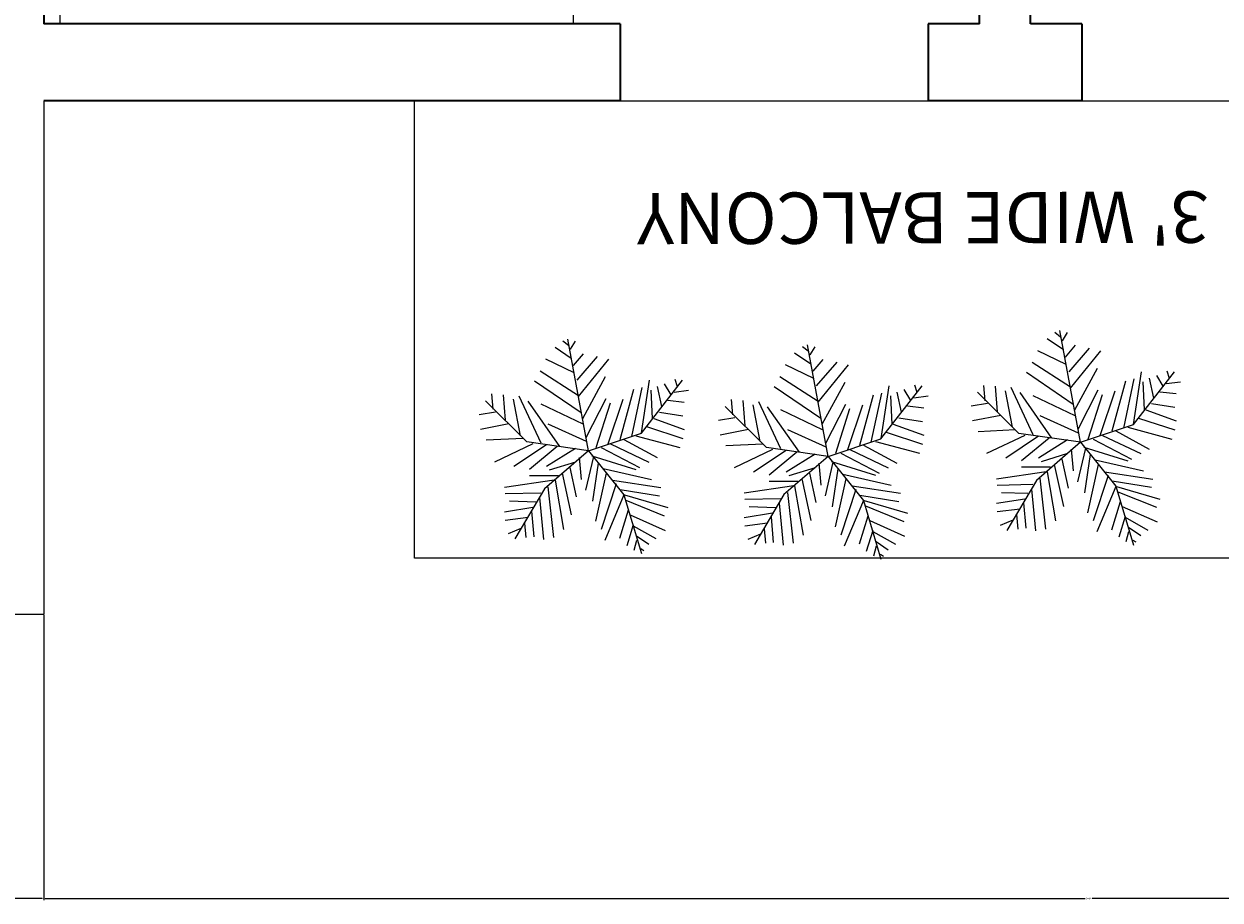
# Model space of a CAD drawing. Units: inches. Extents: x 4159 to 4826, y 299 to 1026.
# Tile 28 of 37: x 4546 to 4685, y 299 to 401. Entities that reach past the tile are written whole.
import ezdxf

# ---------------------------------------------------------------- set-up
doc = ezdxf.new("R2010")
doc.units = ezdxf.units.IN
for name, color, linetype, lineweight in [('A-ANNO-DIMS', 2, 'Continuous', 18), ('A-AREA-IDEN', 7, 'Continuous', 18), ('A-FLOR-BALC', 7, 'Continuous', 25), ('A-FLOR-STRS', 3, 'Continuous', 25), ('A-FURN', 8, 'Continuous', 18), ('A-WALL', 7, 'Continuous', 35), ('L-PLNT', 94, 'Continuous', 13)]:
    doc.layers.add(name, color=color, linetype=linetype, lineweight=lineweight)
doc.styles.get("Standard").update_dxf_attribs({"font": 'arial.ttf'})
doc.dimstyles.get("Standard").update_dxf_attribs({"dimtxt": 0.18, "dimasz": 0.18, "dimexe": 0.18, "dimexo": 0.0625, "dimgap": 0.09, "dimtad": 0, "dimtih": 1, "dimtoh": 1, "dimdec": 4, "dimzin": 0, "dimdsep": 46, "dimtxsty": 'Standard', "dimcen": 0.09, "dimadec": 0, "dimazin": 0, "dimtfac": 1, "dimtdec": 4, "dimtofl": 0, "dimtmove": 0, "dimatfit": 3, "dimfxl": 1, "dimtolj": 1, "dimtzin": 0, "dimarcsym": 0})

# ---------------------------------------------------------------- blocks, each defined once
blk = doc.blocks.new('Bed - Queen')
for p, q in [((0, -80.00003), (0, 0)), ((0, 0), (59.99999, 0)), ((59.99999, 0), (59.99999, -80.00003)), ((7.99999, -1.2), (28.79998, -1.2)), ((7.99999, -14.4), (7.99999, -1.2)), ((28.79998, -1.2), (28.79998, -14.4)), ((31.19999, -1.2), (51.99999, -1.2)), ((31.19999, -14.4), (31.19999, -1.2)), ((51.99999, -1.2), (51.99999, -16.4)), ((0, -14.4), (44.8, -14.4)), ((59.99999, -29.6), (44.8, -14.4)), ((44.8, -14.4), (44.8, -29.6)), ((51.99999, -16.4), (46.79936, -16.4)), ((44.8, -16.8), (0, -16.8)), ((44.8, -29.6), (59.99999, -29.6)), ((59.99999, -80.00003), (0, -80.00003))]:
    blk.add_line(p, q)
blk = doc.blocks.new('*U12')
for p, q in [((-10.186, 53.64), (-13.084, 55.962)), ((0, 0), (-10.5, 57)), ((-9.099, 51.782), (-6.563, 55.962)), ((-8.737, 47.138), (-17.069, 52.711)), ((-7.65, 43.423), (-2.578, 49.46)), ((-7.288, 39.707), (-21.778, 46.673)), ((-5.839, 35.992), (4.667, 48.067)), ((-5.114, 27.632), (10.463, 46.673)), ((-5.114, 28.097), (-24.676, 40.636)), ((-2.941, 16.486), (8.652, 37.85)), ((-3.665, 19.273), (-27.574, 35.527)), ((16.259, 5.805), (23.142, 31.348)), ((22.055, 7.198), (27.489, 32.277)), ((27, 9), (48, 36)), ((27.127, 9.056), (31.112, 35.992)), ((31.836, 30.883), (32.561, 16.486)), ((35.096, 32.741), (37.27, 22.524)), ((38.719, 34.134), (41.979, 28.561)), ((43.791, 29.954), (51.036, 30.883)), ((44.153, 36.456), (45.239, 32.741)), ((-31.5, 4.5), (-52.5, 25.5)), ((-48.585, 21.131), (-49.309, 29.026)), ((-43.513, 28.561), (-42.427, 15.558)), ((-38.442, 26.239), (-34.819, 7.663)), ((-35.544, 28.097), (-24.314, 3.947)), ((-14.533, 2.09), (-30.834, 25.31)), ((-1.129, 6.734), (9.014, 26.704)), ((10.101, 3.483), (17.708, 26.239)), ((40.53, 25.775), (48.862, 24.846)), ((-47.498, 19.737), (-55.83, 18.344)), ((-24.314, 23.917), (-2.941, 13.7)), ((3.942, 1.625), (11.187, 24.381)), ((36.183, 19.737), (48.137, 17.88)), ((-40.615, 13.7), (-55.105, 10.913)), ((-20.691, 13.7), (-1.129, 4.876)), ((29.662, 12.307), (48.137, 6.269)), ((33.285, 16.486), (48.862, 10.913)), ((-33.37, 6.269), (-52.207, 5.34)), ((0, 0), (27, 9)), ((24.229, 7.663), (46.688, 1.625)), ((-28.299, 3.483), (-47.86, -5.805)), ((-21.416, 3.018), (-38.079, -8.128)), ((0, 0), (-31.5, 4.5)), ((-15.982, 2.09), (-30.11, -9.521)), ((0, 0), (-22.5, -19.5)), ((-6.563, 1.161), (-21.416, -8.128)), ((0, 0), (18, -22.5)), ((6.478, 1.625), (26.04, -8.592)), ((11.187, 3.483), (30.749, -5.805)), ((18.07, 5.805), (35.096, -3.483)), ((-6.563, -5.805), (-19.967, -9.985)), ((-4.752, -3.483), (-3.665, -14.629)), ((2.493, -3.019), (-1.491, -20.202)), ((1.769, -2.555), (24.229, -9.521)), ((-13.446, -11.378), (-8.737, -32.741)), ((-9.461, -8.592), (-6.201, -23.453)), ((5.029, -6.27), (2.131, -25.775)), ((9.014, -11.378), (3.58, -35.992)), ((7.565, -9.056), (32.198, -14.629)), ((-17.431, -15.094), (-42.789, -18.809)), ((-15.257, -12.772), (-30.11, -12.772)), ((-17.069, -15.094), (-12.721, -40.172)), ((14.085, -16.951), (6.478, -40.172)), ((12.274, -15.094), (36.907, -18.809)), ((-24.314, -21.596), (-42.427, -22.06)), ((-22.5, -19.5), (-37.5, -45)), ((-25.038, -23.918), (-22.865, -45.281)), ((-20.691, -18.345), (-17.793, -44.352)), ((18.07, -22.524), (8.289, -45.745)), ((16.259, -19.738), (36.183, -22.989)), ((18, -22.5), (27, -52.5)), ((18.433, -22.524), (40.53, -29.026)), ((-28.299, -29.026), (-42.789, -31.348)), ((-26.849, -26.24), (-40.253, -25.775)), ((20.244, -30.419), (15.897, -44.816)), ((19.157, -25.311), (38.719, -33.206)), ((-30.834, -34.135), (-42.427, -35.528)), ((-29.023, -30.884), (-27.936, -43.887)), ((21.331, -32.741), (39.081, -40.636)), ((-34.457, -39.708), (-40.978, -42.494)), ((-32.646, -36.921), (-31.921, -44.352)), ((22.78, -37.85), (19.519, -48.532)), ((22.78, -38.314), (34.372, -44.816)), ((24.591, -45.745), (23.142, -50.854)), ((24.591, -43.423), (30.749, -47.603)), ((26.764, -49.925), (28.213, -50.854))]:
    blk.add_line(p, q)
blk = doc.blocks.new('*D47')
at = {"layer": 'A-ANNO-DIMS', "color": 0, "lineweight": -2, "transparency": 16777216}
for p, q in [((4447.31, 332.13), (4447.31, 298.77)), ((4547.89, 332.13), (4547.89, 298.77)), ((4447.49, 298.95), (4497.14, 298.95)), ((4547.71, 298.95), (4498.06, 298.95))]:
    blk.add_line(p, q, dxfattribs=at)
at = {"layer": 'A-ANNO-DIMS', "color": 0, "transparency": 16777216}
for points in [[(4447.49, 298.98), (4447.49, 298.92), (4447.31, 298.95)], [(4547.71, 298.98), (4547.71, 298.92), (4547.89, 298.95)]]:
    blk.add_solid(points, dxfattribs=at)
at = {"layer": 'Defpoints', "color": 0, "transparency": 16777216}
for p in [(4447.31, 332.2), (4547.89, 332.2), (4547.89, 298.95)]:
    blk.add_point(p, dxfattribs=at)
at = {"layer": 'A-ANNO-DIMS', "color": 0, "transparency": 16777216, "insert": (4497.6, 298.95), "char_height": 0.18, "attachment_point": 5}
blk.add_mtext('\\A1;100.58', dxfattribs=at)
blk = doc.blocks.new('*D48')
at = {"layer": 'A-ANNO-DIMS', "color": 0, "lineweight": -2, "transparency": 16777216}
for p, q in [((4792.31, 392.19), (4792.31, 298.77)), ((4547.89, 332.13), (4547.89, 298.77)), ((4548.07, 298.95), (4669.7, 298.95)), ((4792.13, 298.95), (4670.49, 298.95))]:
    blk.add_line(p, q, dxfattribs=at)
at = {"layer": 'A-ANNO-DIMS', "color": 0, "transparency": 16777216}
for points in [[(4548.07, 298.98), (4548.07, 298.92), (4547.89, 298.95)], [(4792.13, 298.98), (4792.13, 298.92), (4792.31, 298.95)]]:
    blk.add_solid(points, dxfattribs=at)
at = {"layer": 'Defpoints', "color": 0, "transparency": 16777216}
for p in [(4792.31, 392.25), (4547.89, 332.2), (4792.31, 298.95)]:
    blk.add_point(p, dxfattribs=at)
at = {"layer": 'A-ANNO-DIMS', "color": 0, "transparency": 16777216, "insert": (4670.1, 298.95), "char_height": 0.18, "attachment_point": 5}
blk.add_mtext('\\A1;244.4', dxfattribs=at)

msp = doc.modelspace()

# ---------------------------------------------------------------- linework, layer by layer
at = {"layer": 'A-FLOR-BALC'}
msp.add_lwpolyline([(4591.233, 392.254), (4718.606, 392.254), (4718.606, 338.75), (4591.233, 338.75)], close=True, dxfattribs=at)
at = {"layer": 'A-FLOR-STRS'}
for p in [(4547.889, 392.254), (4447.31, 332.195)]:
    msp.add_line(p, (4547.889, 332.195), dxfattribs=at)
at = {"layer": 'A-WALL'}
for p, q in [((4547.889, 533.254), (4547.889, 401.254)), ((4657.31, 401.254), (4657.31, 533.254)), ((4663.31, 401.254), (4663.31, 533.254)), ((4615.31, 401.254), (4547.889, 401.254)), ((4615.31, 401.254), (4547.889, 401.254)), ((4615.31, 401.254), (4615.31, 392.254)), ((4657.31, 401.254), (4651.31, 401.254)), ((4657.31, 401.254), (4651.31, 401.254)), ((4651.31, 401.254), (4651.31, 392.254)), ((4669.31, 401.254), (4663.31, 401.254)), ((4669.31, 401.254), (4663.31, 401.254)), ((4669.31, 401.254), (4669.31, 392.254)), ((4615.31, 392.254), (4547.889, 392.254)), ((4669.31, 392.254), (4651.31, 392.254))]:
    msp.add_line(p, q, dxfattribs=at)

# ---------------------------------------------------------------- block references
at = {"layer": 'A-FURN', "rotation": 180}
msp.add_blockref('Bed - Queen', (4609.814, 401.246), dxfattribs=at)
at = {"layer": 'L-PLNT', "xscale": 0.2292012274639507, "yscale": 0.2292012274639507, "zscale": 0.2292012274639507}
for p in [(4669.136, 352.322), (4611.593, 351.328), (4639.618, 350.665)]:
    msp.add_blockref('*U12', p, dxfattribs=at)

# ---------------------------------------------------------------- texts
at = {"layer": 'A-AREA-IDEN'}
msp.add_text("3' WIDE BALCONY", height=6, rotation=180.15208, dxfattribs=at).set_placement((4684.147, 381.658))

# ---------------------------------------------------------------- dimensions: what is measured, and where the dimension line sits
at = {"layer": 'A-ANNO-DIMS'}
for base, p1, p2, override, picture, middle in [((4792.31, 298.945), (4547.889, 332.195), (4792.31, 392.254), {"dimdec": 1, "dimlfac": 1, "dimrnd": 0, "dimzin": 0, "dimdsep": 46, "dimlunit": 2}, '*D48', (4670.1, 298.945)), ((4547.889, 298.945), (4447.31, 332.195), (4547.889, 332.195), {"dimdec": 2, "dimlfac": 1, "dimrnd": 0, "dimzin": 0, "dimdsep": 46, "dimlunit": 2}, '*D47', (4497.6, 298.945))]:
    dim = msp.add_linear_dim(base=base, p1=p1, p2=p2, dimstyle='Standard', override=override, dxfattribs=at)
    dim.commit()
    dim.dimension.update_dxf_attribs({"geometry": picture, "text_midpoint": middle})

doc.saveas('drawing.dxf')
